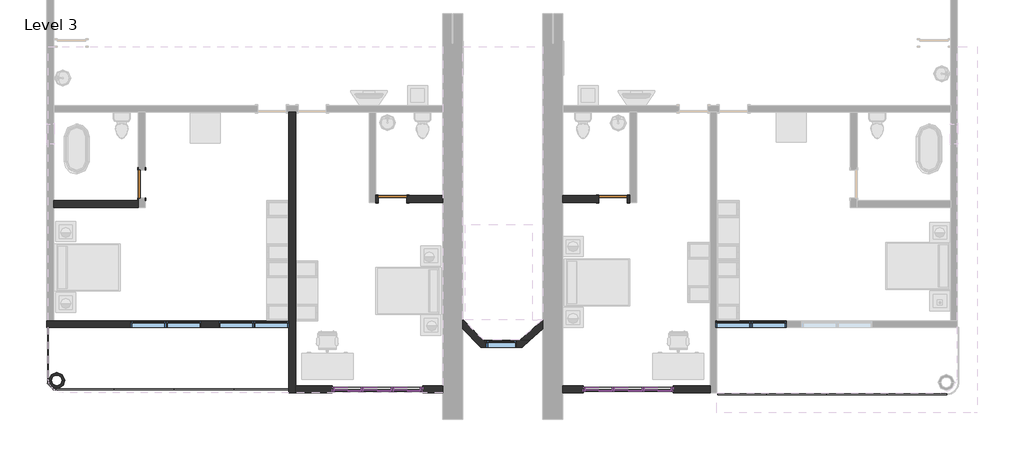
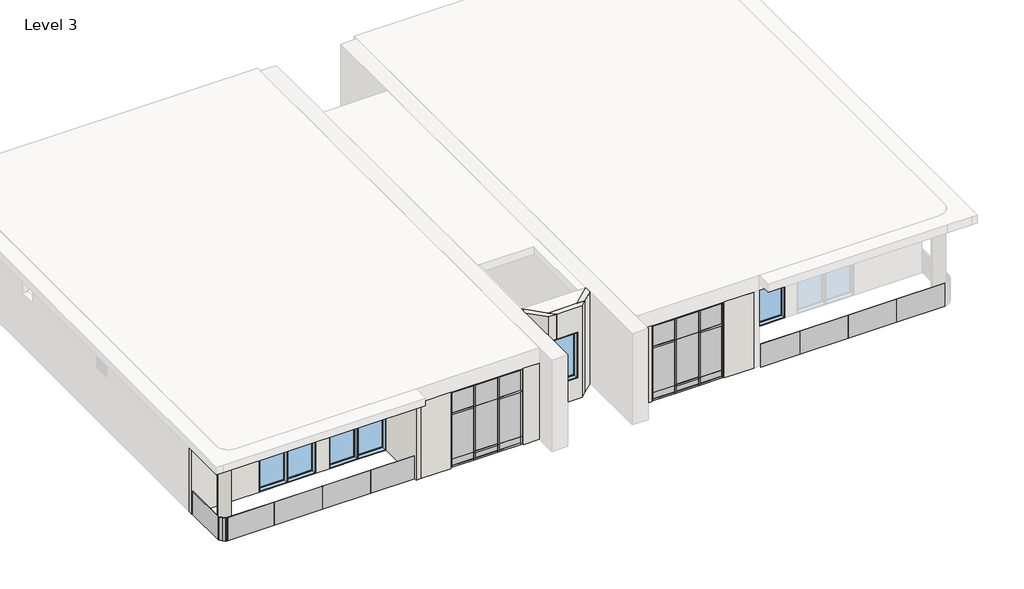
# One storey, part 1 of 3: 42 members, 31 plates, 14 walls, 7 windows, 3 doors.
"""IFC4 building model written with IfcOpenShell, lengths in millimetres."""

from ifc_helpers import new_model, si_unit, point, frame, frame_2d, origin, place, context, project, spatial, polyline, circle_curve, trimmed, segment, composite_curve, outline, extrude, faceted_brep, transform, mapped, element, save
from components import door_2703ae13, door_10fd3a06, member_c17f1be2, member_ad567e07, member_d2e7e466, member_7db1855a, member_75d1e245, member_d60e8053, member_3c3dc66a, member_2fae0574, member_410c6227, member_73c23c35, system_panel_glazed_38d54ecf, system_panel_glazed_fbb6c980, system_panel_glazed_4137532c, system_panel_glazed_6230de04, system_panel_glazed_a79f7f85, system_panel_glazed_9a5ea490, system_panel_glazed_95be5de7, system_panel_glazed_1e00a1c5, system_panel_glazed_ffe51582, system_panel_glazed_8f95e3f6, system_panel_glazed_836907cd, system_panel_glazed_688a65a2, system_panel_glazed_c1a1c740, system_panel_glazed_22bcd51f, window_9a779fa2, window_1a213a25

model = new_model("IFC4")

# Units and contexts
model_context = context("Model", 3, world=origin())
ifc_project = project(units=[si_unit("LENGTHUNIT", "METRE", prefix="MILLI")], contexts=[model_context])

# Site, building, storey
site = spatial("IfcSite", under=ifc_project)
building = spatial("IfcBuilding", under=site)
storey = spatial("IfcBuildingStorey", under=building, Name="Level 3", Elevation=7315.2)

# Doors
placement = place(None, origin())
door_shape = door_2703ae13(model_context)
element("IfcDoor", 1, ObjectType="Door-Single-Panel.0001 : 34\" x 80\"", at=placement, inside=storey, context=model_context, shape_type="MappedRepresentation", body=[
    mapped(door_shape, transform((-15759.6487704, -441.9241442, 7315.2), x_axis=(0.0, -1.0, 0.0), y_axis=(1.0, 0.0, 0.0), z_axis=(0.0, 0.0, 1.0))),
])
element("IfcDoor", 2, ObjectType="Door-Single-Panel.0001 : 34\" x 80\"", at=placement, inside=storey, context=model_context, shape_type="MappedRepresentation", body=[
    mapped(door_shape, transform((-8139.6487704, -899.1241442, 7315.2), x_axis=(-1.0, 0.0, 0.0), y_axis=(0.0, -1.0, 0.0), z_axis=(0.0, 0.0, 1.0))),
])
door_2_shape = door_10fd3a06(model_context)
element("IfcDoor", 3, ObjectType="Door-Single-Panel.0001 : 34\" x 80\"", at=placement, inside=storey, context=model_context, shape_type="MappedRepresentation", body=[
    mapped(door_2_shape, transform((-1434.0487704, -899.1241442, 7315.2), x_axis=(1.0, 0.0, 0.0), y_axis=(0.0, 1.0, 0.0), z_axis=(0.0, 0.0, 1.0))),
])

# Members
member_shape = member_c17f1be2(model_context)
element("IfcMember", 4, ObjectType="Rectangular Mullion : 2.5\" x 5\" rectangular", at=placement, inside=storey, context=model_context, shape_type="MappedRepresentation", body=[
    mapped(member_shape, transform((-9904.9487704, -6690.3241442, 10363.2), x_axis=(0.0, 0.0, 1.0), y_axis=(0.0, 1.0, 0.0), z_axis=(-1.0, 0.0, 0.0))),
])
element("IfcMember", 5, ObjectType="Rectangular Mullion : 2.5\" x 5\" rectangular", at=placement, inside=storey, context=model_context, shape_type="MappedRepresentation", body=[
    mapped(member_shape, transform((-8107.8987704, -6690.3241442, 10363.2), x_axis=(0.0, 0.0, 1.0), y_axis=(0.0, 1.0, 0.0), z_axis=(-1.0, 0.0, 0.0))),
])
element("IfcMember", 6, ObjectType="Rectangular Mullion : 2.5\" x 5\" rectangular", at=placement, inside=storey, context=model_context, shape_type="MappedRepresentation", body=[
    mapped(member_shape, transform((-2284.9487704, -6690.3241442, 10363.2), x_axis=(0.0, 0.0, 1.0), y_axis=(0.0, 1.0, 0.0), z_axis=(-1.0, 0.0, 0.0))),
])
element("IfcMember", 7, ObjectType="Rectangular Mullion : 2.5\" x 5\" rectangular", at=placement, inside=storey, context=model_context, shape_type="MappedRepresentation", body=[
    mapped(member_shape, transform((-487.8987704, -6690.3241442, 10363.2), x_axis=(0.0, 0.0, 1.0), y_axis=(0.0, 1.0, 0.0), z_axis=(-1.0, 0.0, 0.0))),
])
element("IfcMember", 8, ObjectType="Rectangular Mullion : 2.5\" x 5\" rectangular", at=placement, inside=storey, context=model_context, shape_type="MappedRepresentation", body=[
    mapped(member_shape, transform((-7288.7487704, -6690.3241442, 7315.2), x_axis=(0.0, 0.0, -1.0), y_axis=(0.0, 1.0, 0.0), z_axis=(1.0, 0.0, 0.0))),
])
element("IfcMember", 9, ObjectType="Rectangular Mullion : 2.5\" x 5\" rectangular", at=placement, inside=storey, context=model_context, shape_type="MappedRepresentation", body=[
    mapped(member_shape, transform((-9085.7987704, -6690.3241442, 7315.2), x_axis=(0.0, 0.0, -1.0), y_axis=(0.0, 1.0, 0.0), z_axis=(1.0, 0.0, 0.0))),
])
element("IfcMember", 10, ObjectType="Rectangular Mullion : 2.5\" x 5\" rectangular", at=placement, inside=storey, context=model_context, shape_type="MappedRepresentation", body=[
    mapped(member_shape, transform((331.2512296, -6690.3241442, 7315.2), x_axis=(0.0, 0.0, -1.0), y_axis=(0.0, 1.0, 0.0), z_axis=(1.0, 0.0, 0.0))),
])
element("IfcMember", 11, ObjectType="Rectangular Mullion : 2.5\" x 5\" rectangular", at=placement, inside=storey, context=model_context, shape_type="MappedRepresentation", body=[
    mapped(member_shape, transform((-1465.7987704, -6690.3241442, 7315.2), x_axis=(0.0, 0.0, -1.0), y_axis=(0.0, 1.0, 0.0), z_axis=(1.0, 0.0, 0.0))),
])
member_2_shape = member_ad567e07(model_context)
element("IfcMember", 12, ObjectType="Rectangular Mullion : 2.5\" x 5\" rectangular", at=placement, inside=storey, context=model_context, shape_type="MappedRepresentation", body=[
    mapped(member_2_shape, transform((-8107.8987704, -6690.3241442, 9448.8), x_axis=(0.0, 0.0, 1.0), y_axis=(0.0, 1.0, 0.0), z_axis=(-1.0, 0.0, 0.0))),
])
element("IfcMember", 13, ObjectType="Rectangular Mullion : 2.5\" x 5\" rectangular", at=placement, inside=storey, context=model_context, shape_type="MappedRepresentation", body=[
    mapped(member_2_shape, transform((-9904.9487704, -6690.3241442, 9448.8), x_axis=(0.0, 0.0, 1.0), y_axis=(0.0, 1.0, 0.0), z_axis=(-1.0, 0.0, 0.0))),
])
element("IfcMember", 14, ObjectType="Rectangular Mullion : 2.5\" x 5\" rectangular", at=placement, inside=storey, context=model_context, shape_type="MappedRepresentation", body=[
    mapped(member_2_shape, transform((-487.8987704, -6690.3241442, 9448.8), x_axis=(0.0, 0.0, 1.0), y_axis=(0.0, 1.0, 0.0), z_axis=(-1.0, 0.0, 0.0))),
])
element("IfcMember", 15, ObjectType="Rectangular Mullion : 2.5\" x 5\" rectangular", at=placement, inside=storey, context=model_context, shape_type="MappedRepresentation", body=[
    mapped(member_2_shape, transform((-2284.9487704, -6690.3241442, 9448.8), x_axis=(0.0, 0.0, 1.0), y_axis=(0.0, 1.0, 0.0), z_axis=(-1.0, 0.0, 0.0))),
])
member_3_shape = member_d2e7e466(model_context)
element("IfcMember", 16, ObjectType="Rectangular Mullion : 2.5\" x 5\" rectangular", at=placement, inside=storey, context=model_context, shape_type="MappedRepresentation", body=[
    mapped(member_3_shape, transform((-8171.3987704, -6690.3241442, 7315.2), x_axis=(0.0, 0.0, -1.0), y_axis=(0.0, 1.0, 0.0), z_axis=(1.0, 0.0, 0.0))),
])
element("IfcMember", 17, ObjectType="Rectangular Mullion : 2.5\" x 5\" rectangular", at=placement, inside=storey, context=model_context, shape_type="MappedRepresentation", body=[
    mapped(member_3_shape, transform((-551.3987704, -6690.3241442, 7315.2), x_axis=(0.0, 0.0, -1.0), y_axis=(0.0, 1.0, 0.0), z_axis=(1.0, 0.0, 0.0))),
])
member_4_shape = member_7db1855a(model_context)
element("IfcMember", 18, ObjectType="Rectangular Mullion : 2.5\" x 5\" rectangular", at=placement, inside=storey, context=model_context, shape_type="MappedRepresentation", body=[
    mapped(member_4_shape, transform((-9022.2987704, -6690.3241442, 7620.0), x_axis=(0.0, 0.0, 1.0), y_axis=(0.0, 1.0, 0.0), z_axis=(-1.0, 0.0, 0.0))),
])
element("IfcMember", 19, ObjectType="Rectangular Mullion : 2.5\" x 5\" rectangular", at=placement, inside=storey, context=model_context, shape_type="MappedRepresentation", body=[
    mapped(member_4_shape, transform((-1402.2987704, -6690.3241442, 7620.0), x_axis=(0.0, 0.0, 1.0), y_axis=(0.0, 1.0, 0.0), z_axis=(-1.0, 0.0, 0.0))),
])
element("IfcMember", 20, ObjectType="Rectangular Mullion : 2.5\" x 5\" rectangular", at=placement, inside=storey, context=model_context, shape_type="MappedRepresentation", body=[
    mapped(member_3_shape, transform((-9022.2987704, -6690.3241442, 10363.2), x_axis=(0.0, 0.0, 1.0), y_axis=(0.0, 1.0, 0.0), z_axis=(-1.0, 0.0, 0.0))),
])
element("IfcMember", 21, ObjectType="Rectangular Mullion : 2.5\" x 5\" rectangular", at=placement, inside=storey, context=model_context, shape_type="MappedRepresentation", body=[
    mapped(member_3_shape, transform((-1402.2987704, -6690.3241442, 10363.2), x_axis=(0.0, 0.0, 1.0), y_axis=(0.0, 1.0, 0.0), z_axis=(-1.0, 0.0, 0.0))),
])
member_5_shape = member_75d1e245(model_context)
element("IfcMember", 22, ObjectType="Rectangular Mullion : 2.5\" x 5\" rectangular", at=placement, inside=storey, context=model_context, shape_type="MappedRepresentation", body=[
    mapped(member_5_shape, transform((-8139.6487704, -6690.3241442, 7315.2), x_axis=(-1.0, 0.0, 0.0), y_axis=(0.0, 1.0, 0.0), z_axis=(0.0, 0.0, -1.0))),
])
element("IfcMember", 23, ObjectType="Rectangular Mullion : 2.5\" x 5\" rectangular", at=placement, inside=storey, context=model_context, shape_type="MappedRepresentation", body=[
    mapped(member_5_shape, transform((-9054.0487704, -6690.3241442, 7315.2), x_axis=(-1.0, 0.0, 0.0), y_axis=(0.0, 1.0, 0.0), z_axis=(0.0, 0.0, -1.0))),
])
element("IfcMember", 24, ObjectType="Rectangular Mullion : 2.5\" x 5\" rectangular", at=placement, inside=storey, context=model_context, shape_type="MappedRepresentation", body=[
    mapped(member_5_shape, transform((-519.6487704, -6690.3241442, 7315.2), x_axis=(-1.0, 0.0, 0.0), y_axis=(0.0, 1.0, 0.0), z_axis=(0.0, 0.0, -1.0))),
])
element("IfcMember", 25, ObjectType="Rectangular Mullion : 2.5\" x 5\" rectangular", at=placement, inside=storey, context=model_context, shape_type="MappedRepresentation", body=[
    mapped(member_5_shape, transform((-1434.0487704, -6690.3241442, 7315.2), x_axis=(-1.0, 0.0, 0.0), y_axis=(0.0, 1.0, 0.0), z_axis=(0.0, 0.0, -1.0))),
])
member_6_shape = member_d60e8053(model_context)
element("IfcMember", 26, ObjectType="Rectangular Mullion : 2.5\" x 5\" rectangular", at=placement, inside=storey, context=model_context, shape_type="MappedRepresentation", body=[
    mapped(member_6_shape, transform((-8139.6487704, -6690.3241442, 7620.0), x_axis=(-1.0, 0.0, 0.0), y_axis=(0.0, 1.0, 0.0), z_axis=(0.0, 0.0, -1.0))),
])
element("IfcMember", 27, ObjectType="Rectangular Mullion : 2.5\" x 5\" rectangular", at=placement, inside=storey, context=model_context, shape_type="MappedRepresentation", body=[
    mapped(member_6_shape, transform((-9054.0487704, -6690.3241442, 7620.0), x_axis=(-1.0, 0.0, 0.0), y_axis=(0.0, 1.0, 0.0), z_axis=(0.0, 0.0, -1.0))),
])
element("IfcMember", 28, ObjectType="Rectangular Mullion : 2.5\" x 5\" rectangular", at=placement, inside=storey, context=model_context, shape_type="MappedRepresentation", body=[
    mapped(member_6_shape, transform((-519.6487704, -6690.3241442, 7620.0), x_axis=(-1.0, 0.0, 0.0), y_axis=(0.0, 1.0, 0.0), z_axis=(0.0, 0.0, -1.0))),
])
element("IfcMember", 29, ObjectType="Rectangular Mullion : 2.5\" x 5\" rectangular", at=placement, inside=storey, context=model_context, shape_type="MappedRepresentation", body=[
    mapped(member_6_shape, transform((-1434.0487704, -6690.3241442, 7620.0), x_axis=(-1.0, 0.0, 0.0), y_axis=(0.0, 1.0, 0.0), z_axis=(0.0, 0.0, -1.0))),
])
member_7_shape = member_3c3dc66a(model_context)
element("IfcMember", 30, ObjectType="Rectangular Mullion : 2.5\" x 5\" rectangular", at=placement, inside=storey, context=model_context, shape_type="MappedRepresentation", body=[
    mapped(member_7_shape, transform((-9968.4487704, -6690.3241442, 7315.2), x_axis=(-1.0, 0.0, 0.0), y_axis=(0.0, 1.0, 0.0), z_axis=(0.0, 0.0, -1.0))),
])
element("IfcMember", 31, ObjectType="Rectangular Mullion : 2.5\" x 5\" rectangular", at=placement, inside=storey, context=model_context, shape_type="MappedRepresentation", body=[
    mapped(member_7_shape, transform((-2348.4487704, -6690.3241442, 7315.2), x_axis=(-1.0, 0.0, 0.0), y_axis=(0.0, 1.0, 0.0), z_axis=(0.0, 0.0, -1.0))),
])
member_8_shape = member_2fae0574(model_context)
element("IfcMember", 32, ObjectType="Rectangular Mullion : 2.5\" x 5\" rectangular", at=placement, inside=storey, context=model_context, shape_type="MappedRepresentation", body=[
    mapped(member_8_shape, transform((-9968.4487704, -6690.3241442, 7620.0), x_axis=(-1.0, 0.0, 0.0), y_axis=(0.0, 1.0, 0.0), z_axis=(0.0, 0.0, -1.0))),
])
element("IfcMember", 33, ObjectType="Rectangular Mullion : 2.5\" x 5\" rectangular", at=placement, inside=storey, context=model_context, shape_type="MappedRepresentation", body=[
    mapped(member_8_shape, transform((-2348.4487704, -6690.3241442, 7620.0), x_axis=(-1.0, 0.0, 0.0), y_axis=(0.0, 1.0, 0.0), z_axis=(0.0, 0.0, -1.0))),
])
element("IfcMember", 34, ObjectType="Rectangular Mullion : 2.5\" x 5\" rectangular", at=placement, inside=storey, context=model_context, shape_type="MappedRepresentation", body=[
    mapped(member_8_shape, transform((-7225.2487704, -6690.3241442, 9448.8), x_axis=(1.0, 0.0, 0.0), y_axis=(0.0, 1.0, 0.0), z_axis=(0.0, 0.0, 1.0))),
])
element("IfcMember", 35, ObjectType="Rectangular Mullion : 2.5\" x 5\" rectangular", at=placement, inside=storey, context=model_context, shape_type="MappedRepresentation", body=[
    mapped(member_8_shape, transform((394.7512296, -6690.3241442, 9448.8), x_axis=(1.0, 0.0, 0.0), y_axis=(0.0, 1.0, 0.0), z_axis=(0.0, 0.0, 1.0))),
])
element("IfcMember", 36, ObjectType="Rectangular Mullion : 2.5\" x 5\" rectangular", at=placement, inside=storey, context=model_context, shape_type="MappedRepresentation", body=[
    mapped(member_7_shape, transform((-7225.2487704, -6690.3241442, 7620.0), x_axis=(1.0, 0.0, 0.0), y_axis=(0.0, 1.0, 0.0), z_axis=(0.0, 0.0, 1.0))),
])
element("IfcMember", 37, ObjectType="Rectangular Mullion : 2.5\" x 5\" rectangular", at=placement, inside=storey, context=model_context, shape_type="MappedRepresentation", body=[
    mapped(member_7_shape, transform((394.7512296, -6690.3241442, 7620.0), x_axis=(1.0, 0.0, 0.0), y_axis=(0.0, 1.0, 0.0), z_axis=(0.0, 0.0, 1.0))),
])
member_9_shape = member_410c6227(model_context)
element("IfcMember", 38, ObjectType="Rectangular Mullion : 2.5\" x 5\" rectangular", at=placement, inside=storey, context=model_context, shape_type="MappedRepresentation", body=[
    mapped(member_9_shape, transform((-8139.6487704, -6690.3241442, 9448.8), x_axis=(-1.0, 0.0, 0.0), y_axis=(0.0, 1.0, 0.0), z_axis=(0.0, 0.0, -1.0))),
])
element("IfcMember", 39, ObjectType="Rectangular Mullion : 2.5\" x 5\" rectangular", at=placement, inside=storey, context=model_context, shape_type="MappedRepresentation", body=[
    mapped(member_9_shape, transform((-9054.0487704, -6690.3241442, 9448.8), x_axis=(-1.0, 0.0, 0.0), y_axis=(0.0, 1.0, 0.0), z_axis=(0.0, 0.0, -1.0))),
])
element("IfcMember", 40, ObjectType="Rectangular Mullion : 2.5\" x 5\" rectangular", at=placement, inside=storey, context=model_context, shape_type="MappedRepresentation", body=[
    mapped(member_9_shape, transform((-519.6487704, -6690.3241442, 9448.8), x_axis=(-1.0, 0.0, 0.0), y_axis=(0.0, 1.0, 0.0), z_axis=(0.0, 0.0, -1.0))),
])
element("IfcMember", 41, ObjectType="Rectangular Mullion : 2.5\" x 5\" rectangular", at=placement, inside=storey, context=model_context, shape_type="MappedRepresentation", body=[
    mapped(member_9_shape, transform((-1434.0487704, -6690.3241442, 9448.8), x_axis=(-1.0, 0.0, 0.0), y_axis=(0.0, 1.0, 0.0), z_axis=(0.0, 0.0, -1.0))),
])
member_10_shape = member_73c23c35(model_context)
element("IfcMember", 42, ObjectType="Rectangular Mullion : 2.5\" x 5\" rectangular", at=placement, inside=storey, context=model_context, shape_type="MappedRepresentation", body=[
    mapped(member_10_shape, transform((-7225.2487704, -6690.3241442, 10363.2), x_axis=(1.0, 0.0, 0.0), y_axis=(0.0, 1.0, 0.0), z_axis=(0.0, 0.0, 1.0))),
])
element("IfcMember", 43, ObjectType="Rectangular Mullion : 2.5\" x 5\" rectangular", at=placement, inside=storey, context=model_context, shape_type="MappedRepresentation", body=[
    mapped(member_10_shape, transform((394.7512296, -6690.3241442, 10363.2), x_axis=(1.0, 0.0, 0.0), y_axis=(0.0, 1.0, 0.0), z_axis=(0.0, 0.0, 1.0))),
])
element("IfcMember", 44, ObjectType="Rectangular Mullion : 2.5\" x 5\" rectangular", at=placement, inside=storey, context=model_context, shape_type="MappedRepresentation", body=[
    mapped(member_10_shape, transform((-9968.4487704, -6690.3241442, 9448.8), x_axis=(-1.0, 0.0, 0.0), y_axis=(0.0, 1.0, 0.0), z_axis=(0.0, 0.0, -1.0))),
])
element("IfcMember", 45, ObjectType="Rectangular Mullion : 2.5\" x 5\" rectangular", at=placement, inside=storey, context=model_context, shape_type="MappedRepresentation", body=[
    mapped(member_10_shape, transform((-2348.4487704, -6690.3241442, 9448.8), x_axis=(-1.0, 0.0, 0.0), y_axis=(0.0, 1.0, 0.0), z_axis=(0.0, 0.0, -1.0))),
])

# Plates
system_panel_glazed_shape = system_panel_glazed_38d54ecf(model_context)
element("IfcPlate", 46, ObjectType="System Panel : Glazed", at=placement, inside=storey, context=model_context, shape_type="MappedRepresentation", body=[
    mapped(system_panel_glazed_shape, transform((-8596.8487704, -6690.3241442, 7651.75), x_axis=(-1.0, 0.0, 0.0), y_axis=(0.0, -1.0, 0.0), z_axis=(0.0, 0.0, 1.0))),
])
element("IfcPlate", 47, ObjectType="System Panel : Glazed", at=placement, inside=storey, context=model_context, shape_type="MappedRepresentation", body=[
    mapped(system_panel_glazed_shape, transform((-976.8487704, -6690.3241442, 7651.75), x_axis=(-1.0, 0.0, 0.0), y_axis=(0.0, -1.0, 0.0), z_axis=(0.0, 0.0, 1.0))),
])
system_panel_glazed_2_shape = system_panel_glazed_fbb6c980(model_context)
element("IfcPlate", 48, ObjectType="System Panel : Glazed", at=placement, inside=storey, context=model_context, shape_type="MappedRepresentation", body=[
    mapped(system_panel_glazed_2_shape, transform((-8596.8487704, -6690.3241442, 7378.7), x_axis=(-1.0, 0.0, 0.0), y_axis=(0.0, -1.0, 0.0), z_axis=(0.0, 0.0, 1.0))),
])
element("IfcPlate", 49, ObjectType="System Panel : Glazed", at=placement, inside=storey, context=model_context, shape_type="MappedRepresentation", body=[
    mapped(system_panel_glazed_2_shape, transform((-976.8487704, -6690.3241442, 7378.7), x_axis=(-1.0, 0.0, 0.0), y_axis=(0.0, -1.0, 0.0), z_axis=(0.0, 0.0, 1.0))),
])
system_panel_glazed_3_shape = system_panel_glazed_4137532c(model_context)
element("IfcPlate", 50, ObjectType="System Panel : Glazed", at=placement, inside=storey, context=model_context, shape_type="MappedRepresentation", body=[
    mapped(system_panel_glazed_3_shape, transform((-7698.3237704, -6690.3241442, 7378.7), x_axis=(-1.0, 0.0, 0.0), y_axis=(0.0, -1.0, 0.0), z_axis=(0.0, 0.0, 1.0))),
])
element("IfcPlate", 51, ObjectType="System Panel : Glazed", at=placement, inside=storey, context=model_context, shape_type="MappedRepresentation", body=[
    mapped(system_panel_glazed_3_shape, transform((-9495.3737704, -6690.3241442, 7378.7), x_axis=(-1.0, 0.0, 0.0), y_axis=(0.0, -1.0, 0.0), z_axis=(0.0, 0.0, 1.0))),
])
element("IfcPlate", 52, ObjectType="System Panel : Glazed", at=placement, inside=storey, context=model_context, shape_type="MappedRepresentation", body=[
    mapped(system_panel_glazed_3_shape, transform((-78.3237704, -6690.3241442, 7378.7), x_axis=(-1.0, 0.0, 0.0), y_axis=(0.0, -1.0, 0.0), z_axis=(0.0, 0.0, 1.0))),
])
element("IfcPlate", 53, ObjectType="System Panel : Glazed", at=placement, inside=storey, context=model_context, shape_type="MappedRepresentation", body=[
    mapped(system_panel_glazed_3_shape, transform((-1875.3737704, -6690.3241442, 7378.7), x_axis=(-1.0, 0.0, 0.0), y_axis=(0.0, -1.0, 0.0), z_axis=(0.0, 0.0, 1.0))),
])
system_panel_glazed_4_shape = system_panel_glazed_6230de04(model_context)
element("IfcPlate", 54, ObjectType="System Panel : Glazed", at=placement, inside=storey, context=model_context, shape_type="MappedRepresentation", body=[
    mapped(system_panel_glazed_4_shape, transform((-7698.3237704, -6690.3241442, 7620.0), x_axis=(-1.0, 0.0, 0.0), y_axis=(0.0, -1.0, 0.0), z_axis=(0.0, 0.0, 1.0))),
])
element("IfcPlate", 55, ObjectType="System Panel : Glazed", at=placement, inside=storey, context=model_context, shape_type="MappedRepresentation", body=[
    mapped(system_panel_glazed_4_shape, transform((-9495.3737704, -6690.3241442, 7620.0), x_axis=(-1.0, 0.0, 0.0), y_axis=(0.0, -1.0, 0.0), z_axis=(0.0, 0.0, 1.0))),
])
element("IfcPlate", 56, ObjectType="System Panel : Glazed", at=placement, inside=storey, context=model_context, shape_type="MappedRepresentation", body=[
    mapped(system_panel_glazed_4_shape, transform((-78.3237704, -6690.3241442, 7620.0), x_axis=(-1.0, 0.0, 0.0), y_axis=(0.0, -1.0, 0.0), z_axis=(0.0, 0.0, 1.0))),
])
element("IfcPlate", 57, ObjectType="System Panel : Glazed", at=placement, inside=storey, context=model_context, shape_type="MappedRepresentation", body=[
    mapped(system_panel_glazed_4_shape, transform((-1875.3737704, -6690.3241442, 7620.0), x_axis=(-1.0, 0.0, 0.0), y_axis=(0.0, -1.0, 0.0), z_axis=(0.0, 0.0, 1.0))),
])
system_panel_glazed_5_shape = system_panel_glazed_a79f7f85(model_context)
element("IfcPlate", 58, ObjectType="System Panel : Glazed", at=placement, inside=storey, context=model_context, shape_type="MappedRepresentation", body=[
    mapped(system_panel_glazed_5_shape, transform((-7698.3237704, -6690.3241442, 9480.55), x_axis=(-1.0, 0.0, 0.0), y_axis=(0.0, -1.0, 0.0), z_axis=(0.0, 0.0, 1.0))),
])
element("IfcPlate", 59, ObjectType="System Panel : Glazed", at=placement, inside=storey, context=model_context, shape_type="MappedRepresentation", body=[
    mapped(system_panel_glazed_5_shape, transform((-9495.3737704, -6690.3241442, 9480.55), x_axis=(-1.0, 0.0, 0.0), y_axis=(0.0, -1.0, 0.0), z_axis=(0.0, 0.0, 1.0))),
])
element("IfcPlate", 60, ObjectType="System Panel : Glazed", at=placement, inside=storey, context=model_context, shape_type="MappedRepresentation", body=[
    mapped(system_panel_glazed_5_shape, transform((-78.3237704, -6690.3241442, 9480.55), x_axis=(-1.0, 0.0, 0.0), y_axis=(0.0, -1.0, 0.0), z_axis=(0.0, 0.0, 1.0))),
])
element("IfcPlate", 61, ObjectType="System Panel : Glazed", at=placement, inside=storey, context=model_context, shape_type="MappedRepresentation", body=[
    mapped(system_panel_glazed_5_shape, transform((-1875.3737704, -6690.3241442, 9480.55), x_axis=(-1.0, 0.0, 0.0), y_axis=(0.0, -1.0, 0.0), z_axis=(0.0, 0.0, 1.0))),
])
system_panel_glazed_6_shape = system_panel_glazed_9a5ea490(model_context)
element("IfcPlate", 62, ObjectType="System Panel : Glazed", at=placement, inside=storey, context=model_context, shape_type="MappedRepresentation", body=[
    mapped(system_panel_glazed_6_shape, transform((-8596.8487704, -6690.3241442, 9448.8), x_axis=(-1.0, 0.0, 0.0), y_axis=(0.0, -1.0, 0.0), z_axis=(0.0, 0.0, 1.0))),
])
element("IfcPlate", 63, ObjectType="System Panel : Glazed", at=placement, inside=storey, context=model_context, shape_type="MappedRepresentation", body=[
    mapped(system_panel_glazed_6_shape, transform((-976.8487704, -6690.3241442, 9448.8), x_axis=(-1.0, 0.0, 0.0), y_axis=(0.0, -1.0, 0.0), z_axis=(0.0, 0.0, 1.0))),
])
system_panel_glazed_7_shape = system_panel_glazed_95be5de7(model_context)
element("IfcPlate", 64, ObjectType="System Panel : Glazed", at=placement, inside=storey, context=model_context, shape_type="MappedRepresentation", body=[
    mapped(system_panel_glazed_7_shape, transform((-15700.8805745, -6723.6923401, 7315.2), x_axis=(1.0, 0.0, 0.0), y_axis=(0.0, 1.0, 0.0), z_axis=(0.0, 0.0, 1.0))),
])
element("IfcPlate", 65, ObjectType="System Panel : Glazed", at=placement, inside=storey, context=model_context, shape_type="MappedRepresentation", body=[
    mapped(system_panel_glazed_7_shape, transform((-13872.0805745, -6723.6923401, 7315.2), x_axis=(1.0, 0.0, 0.0), y_axis=(0.0, 1.0, 0.0), z_axis=(0.0, 0.0, 1.0))),
])
element("IfcPlate", 66, ObjectType="System Panel : Glazed", at=placement, inside=storey, context=model_context, shape_type="MappedRepresentation", body=[
    mapped(system_panel_glazed_7_shape, transform((7793.0620092, -6810.4133646, 7315.2), x_axis=(-1.0, 0.0, 0.0), y_axis=(0.0, -1.0, 0.0), z_axis=(0.0, 0.0, 1.0))),
])
element("IfcPlate", 67, ObjectType="System Panel : Glazed", at=placement, inside=storey, context=model_context, shape_type="MappedRepresentation", body=[
    mapped(system_panel_glazed_7_shape, transform((5964.2620092, -6810.4133646, 7315.2), x_axis=(-1.0, 0.0, 0.0), y_axis=(0.0, -1.0, 0.0), z_axis=(0.0, 0.0, 1.0))),
])
element("IfcPlate", 68, ObjectType="System Panel : Glazed", at=placement, inside=storey, context=model_context, shape_type="MappedRepresentation", body=[
    mapped(system_panel_glazed_7_shape, transform((4135.4620092, -6810.4133646, 7315.2), x_axis=(-1.0, 0.0, 0.0), y_axis=(0.0, -1.0, 0.0), z_axis=(0.0, 0.0, 1.0))),
])
system_panel_glazed_8_shape = system_panel_glazed_1e00a1c5(model_context)
element("IfcPlate", 69, ObjectType="System Panel : Glazed", at=placement, inside=storey, context=model_context, shape_type="MappedRepresentation", body=[
    mapped(system_panel_glazed_8_shape, transform((2484.4620092, -6810.4133646, 7315.2), x_axis=(-1.0, 0.0, 0.0), y_axis=(0.0, -1.0, 0.0), z_axis=(0.0, 0.0, 1.0))),
])
system_panel_glazed_9_shape = system_panel_glazed_ffe51582(model_context)
element("IfcPlate", 70, ObjectType="System Panel : Glazed", at=placement, inside=storey, context=model_context, shape_type="MappedRepresentation", body=[
    mapped(system_panel_glazed_9_shape, transform((-18445.6213429, -6722.1515718, 7315.2), x_axis=(0.7071067811865462, -0.7071067811865488, 0.0), y_axis=(0.7071067811865488, 0.7071067811865462, 0.0), z_axis=(0.0, 0.0, 1.0))),
])
system_panel_glazed_10_shape = system_panel_glazed_8f95e3f6(model_context)
element("IfcPlate", 71, ObjectType="System Panel : Glazed", at=placement, inside=storey, context=model_context, shape_type="MappedRepresentation", body=[
    mapped(system_panel_glazed_10_shape, transform((-18642.5487704, -5667.9741442, 7315.2), x_axis=(0.0, -1.0, 0.0), y_axis=(1.0, 0.0, 0.0), z_axis=(0.0, 0.0, 1.0))),
])
system_panel_glazed_11_shape = system_panel_glazed_836907cd(model_context)
element("IfcPlate", 72, ObjectType="System Panel : Glazed", at=placement, inside=storey, context=model_context, shape_type="MappedRepresentation", body=[
    mapped(system_panel_glazed_11_shape, transform((-18412.3305745, -6723.6923401, 7315.2), x_axis=(1.0, 0.0, 0.0), y_axis=(0.0, 1.0, 0.0), z_axis=(0.0, 0.0, 1.0))),
])
system_panel_glazed_12_shape = system_panel_glazed_688a65a2(model_context)
element("IfcPlate", 73, ObjectType="System Panel : Glazed", at=placement, inside=storey, context=model_context, shape_type="MappedRepresentation", body=[
    mapped(system_panel_glazed_12_shape, transform((-12123.4646725, -6723.6923401, 7315.2), x_axis=(1.0, 0.0, 0.0), y_axis=(0.0, 1.0, 0.0), z_axis=(0.0, 0.0, 1.0))),
])
system_panel_glazed_13_shape = system_panel_glazed_c1a1c740(model_context)
element("IfcPlate", 74, ObjectType="System Panel : Glazed", at=placement, inside=storey, context=model_context, shape_type="MappedRepresentation", body=[
    mapped(system_panel_glazed_13_shape, transform((-17497.9305745, -6723.6923401, 7315.2), x_axis=(1.0, 0.0, 0.0), y_axis=(0.0, 1.0, 0.0), z_axis=(0.0, 0.0, 1.0))),
])
system_panel_glazed_14_shape = system_panel_glazed_22bcd51f(model_context)
element("IfcPlate", 75, ObjectType="System Panel : Glazed", at=placement, inside=storey, context=model_context, shape_type="MappedRepresentation", body=[
    mapped(system_panel_glazed_14_shape, transform((-18593.7021056, -6574.070809, 7315.2), x_axis=(0.7071067811865462, -0.7071067811865488, 0.0), y_axis=(0.7071067811865488, 0.7071067811865462, 0.0), z_axis=(0.0, 0.0, 1.0))),
])
element("IfcPlate", 76, ObjectType="System Panel : Glazed", at=placement, inside=storey, context=model_context, shape_type="MappedRepresentation", body=[
    mapped(system_panel_glazed_14_shape, transform((-18496.0087761, -6671.7641386, 7315.2), x_axis=(0.7071067811865462, -0.7071067811865488, 0.0), y_axis=(0.7071067811865488, 0.7071067811865462, 0.0), z_axis=(0.0, 0.0, 1.0))),
])

# Walls
element("IfcWall", 77, ObjectType="Generic - 3\" green 2", at=placement, inside=storey, context=model_context, shape_type="SweptSolid", body=[
    extrude(outline(composite_curve([segment(polyline([(-18512.3737704, -6418.8616442), (-18588.5737704, -6418.8616442)]), True, "CONTINUOUS"), segment(trimmed(circle_curve(frame_2d((-18347.2737704, -6418.8616442)), 241.3), [point((-18588.5737704, -6418.8616442))], [point((-18105.9737704, -6418.8616442))], False, "CARTESIAN"), True, "CONTINUOUS"), segment(polyline([(-18105.9737704, -6418.8616442), (-18182.1737704, -6418.8616442)]), True, "CONTINUOUS"), segment(trimmed(circle_curve(frame_2d((-18347.2737704, -6418.8616442)), 165.1), [point((-18182.1737704, -6418.8616442))], [point((-18512.3737704, -6418.8616442))], True, "CARTESIAN"), True, "CONTINUOUS")], self_intersect=False)), frame((0.0, 0.0, 7315.2), z_axis=(0.0, 0.0, 1.0), x_axis=(1.0, 0.0, 0.0)), (0.0, 0.0, 1.0), 3048.0),
])
element("IfcWall", 78, ObjectType="Generic - 3\" green 2", at=placement, inside=storey, context=model_context, shape_type="SweptSolid", body=[
    extrude(outline(composite_curve([segment(polyline([(-18182.1737704, -6418.8616442), (-18105.9737704, -6418.8616442)]), True, "CONTINUOUS"), segment(trimmed(circle_curve(frame_2d((-18347.2737704, -6418.8616442)), 241.3), [point((-18105.9737704, -6418.8616442))], [point((-18588.5737704, -6418.8616442))], False, "CARTESIAN"), True, "CONTINUOUS"), segment(polyline([(-18588.5737704, -6418.8616442), (-18512.3737704, -6418.8616442)]), True, "CONTINUOUS"), segment(trimmed(circle_curve(frame_2d((-18347.2737704, -6418.8616442)), 165.1), [point((-18512.3737704, -6418.8616442))], [point((-18182.1737704, -6418.8616442))], True, "CARTESIAN"), True, "CONTINUOUS")], self_intersect=False)), frame((0.0, 0.0, 7315.2), z_axis=(0.0, 0.0, 1.0), x_axis=(1.0, 0.0, 0.0)), (0.0, 0.0, 1.0), 3048.0),
])
element("IfcWall", 79, ObjectType="Generic - 8\" cream", at=placement, inside=storey, context=model_context, shape_type="Brep", body=[
    faceted_brep([(-11289.2487704, 1742.4758558, 7315.2), (-11289.2487704, -6791.9241442, 7315.2), (-11289.2487704, -6791.9241442, 10363.2), (-11289.2487704, -4810.7241442, 10363.2), (-11289.2487704, -4607.5241442, 10363.2), (-11289.2487704, 1742.4758558, 10363.2), (-11086.0487704, 1742.4758558, 7315.2), (-11086.0487704, 1742.4758558, 10363.2), (-11086.0487704, -6588.7241442, 10363.2), (-11086.0487704, -6791.9241442, 10363.2), (-11086.0487704, -6791.9241442, 7315.2), (-11086.0487704, -6588.7241442, 7315.2)], [[[0, 1, 2, 3, 4, 5]], [[6, 7, 8, 9, 10, 11]], [[1, 0, 6, 11, 10]], [[5, 4, 3, 2, 9, 8, 7]], [[0, 5, 7, 6]], [[2, 1, 10, 9]]]),
])
element("IfcWall", 80, ObjectType="Generic - 8\" cream", at=placement, inside=storey, context=model_context, shape_type="SweptSolid", body=[
    extrude(outline(polyline([(-18439.3487704, -949.9241442), (-15861.2487704, -949.9241442), (-15861.2487704, -1153.1241442), (-18439.3487704, -1153.1241442), (-18439.3487704, -949.9241442)])), frame((0.0, 0.0, 7315.2), z_axis=(0.0, 0.0, 1.0), x_axis=(1.0, 0.0, 0.0)), (0.0, 0.0, 1.0), 3048.0),
])
element("IfcWall", 81, ObjectType="Generic - 8\" cream", at=placement, inside=storey, context=model_context, shape_type="SweptSolid", body=[
    extrude(outline(polyline([(10363.2, -6615.6487704), (10363.2, -8647.6487704), (7315.2, -8647.6487704), (7315.2, -8571.4487704), (9347.2, -8571.4487704), (9347.2, -7707.8487704), (7315.2, -7707.8487704), (7315.2, -6615.6487704), (10363.2, -6615.6487704)])), frame((0.0, -1000.7241442, 0.0), z_axis=(0.0, 1.0, 0.0), x_axis=(0.0, 0.0, 1.0)), (0.0, 0.0, 1.0), 203.2),
])
element("IfcWall", 82, ObjectType="Generic - 8\" cream", at=placement, inside=storey, context=model_context, shape_type="Brep", body=[
    faceted_brep([(-18642.5487704, -4607.5241442, 10363.2), (-18439.3487704, -4607.5241442, 10363.2), (-11289.2487704, -4607.5241442, 10363.2), (-11289.2487704, -4607.5241442, 10058.4), (-13422.8487704, -4607.5241442, 10058.4), (-13422.8487704, -4607.5241442, 7315.2), (-13956.2487704, -4607.5241442, 7315.2), (-13956.2487704, -4607.5241442, 10058.4), (-16089.8487704, -4607.5241442, 10058.4), (-16089.8487704, -4607.5241442, 7315.2), (-18439.3487704, -4607.5241442, 7315.2), (-18642.5487704, -4607.5241442, 7315.2), (-11289.2487704, -4810.7241442, 10363.2), (-18642.5487704, -4810.7241442, 10363.2), (-18642.5487704, -4810.7241442, 7315.2), (-16089.8487704, -4810.7241442, 7315.2), (-16089.8487704, -4810.7241442, 10058.4), (-13956.2487704, -4810.7241442, 10058.4), (-13956.2487704, -4810.7241442, 7315.2), (-13422.8487704, -4810.7241442, 7315.2), (-13422.8487704, -4810.7241442, 10058.4), (-11289.2487704, -4810.7241442, 10058.4)], [[[0, 1, 2, 3, 4, 5, 6, 7, 8, 9, 10, 11]], [[12, 13, 14, 15, 16, 17, 18, 19, 20, 21]], [[14, 11, 10, 9, 15]], [[5, 19, 18, 6]], [[2, 1, 0, 13, 12]], [[2, 12, 21, 3]], [[0, 11, 14, 13]], [[3, 21, 20, 4]], [[4, 20, 19, 5]], [[17, 7, 6, 18]], [[7, 17, 16, 8]], [[8, 16, 15, 9]]]),
])
element("IfcWall", 83, ObjectType="Generic - 8\" cream", at=placement, inside=storey, context=model_context, shape_type="SweptSolid", body=[
    extrude(outline(polyline([(10363.2, -926.0487704), (10363.2, -2958.0487704), (7315.2, -2958.0487704), (7315.2, -1865.8487704), (9347.2, -1865.8487704), (9347.2, -1002.2487704), (7315.2, -1002.2487704), (7315.2, -926.0487704), (10363.2, -926.0487704)])), frame((0.0, -1000.7241442, 0.0), z_axis=(0.0, 1.0, 0.0), x_axis=(0.0, 0.0, 1.0)), (0.0, 0.0, 1.0), 203.2),
])
element("IfcWall", 84, ObjectType="Generic - 8\" cream", at=placement, inside=storey, context=model_context, shape_type="SweptSolid", body=[
    extrude(outline(polyline([(394.7512296, -6588.7241442), (1512.3512296, -6588.7241442), (1512.3512296, -6791.9241442), (394.7512296, -6791.9241442), (394.7512296, -6588.7241442)])), frame((0.0, 0.0, 7315.2), z_axis=(0.0, 0.0, 1.0), x_axis=(1.0, 0.0, 0.0)), (0.0, 0.0, 1.0), 3048.0),
])
element("IfcWall", 85, ObjectType="Generic - 8\" cream", at=placement, inside=storey, context=model_context, shape_type="SweptSolid", body=[
    extrude(outline(polyline([(-2348.4487704, -6791.9241442), (-2958.0487704, -6791.9241442), (-2958.0487704, -6588.7241442), (-2348.4487704, -6588.7241442), (-2348.4487704, -6791.9241442)])), frame((0.0, 0.0, 7315.2), z_axis=(0.0, 0.0, 1.0), x_axis=(1.0, 0.0, 0.0)), (0.0, 0.0, 1.0), 3048.0),
])
element("IfcWall", 86, ObjectType="Generic - 8\" cream", at=placement, inside=storey, context=model_context, shape_type="SweptSolid", body=[
    extrude(outline(polyline([(-9968.4487704, -6791.9241442), (-11086.0487704, -6791.9241442), (-11086.0487704, -6588.7241442), (-9968.4487704, -6588.7241442), (-9968.4487704, -6791.9241442)])), frame((0.0, 0.0, 7315.2), z_axis=(0.0, 0.0, 1.0), x_axis=(1.0, 0.0, 0.0)), (0.0, 0.0, 1.0), 3048.0),
])
element("IfcWall", 87, ObjectType="Generic - 8\" cream", at=placement, inside=storey, context=model_context, shape_type="SweptSolid", body=[
    extrude(outline(polyline([(-7225.2487704, -6588.7241442), (-6615.6487704, -6588.7241442), (-6615.6487704, -6791.9241442), (-7225.2487704, -6791.9241442), (-7225.2487704, -6588.7241442)])), frame((0.0, 0.0, 7315.2), z_axis=(0.0, 0.0, 1.0), x_axis=(1.0, 0.0, 0.0)), (0.0, 0.0, 1.0), 3048.0),
])
element("IfcWall", 88, ObjectType="Generic - 8\" green", at=placement, inside=storey, context=model_context, shape_type="Brep", body=[
    faceted_brep([(-6006.0487704, -4852.8082422, 7315.2), (-5452.3544276, -5406.502585, 7315.2), (-5452.3544276, -5406.502585, 10972.8), (-6006.0487704, -4852.8082422, 10972.8), (-5164.9862318, -5406.502585, 7315.2), (-5368.1862318, -5203.302585, 7315.2), (-6006.0487704, -4565.4400463, 7315.2), (-6006.0487704, -4565.4400463, 10972.8), (-5368.1862318, -5203.302585, 10972.8), (-5164.9862318, -5406.502585, 10972.8), (-5164.9862318, -5406.502585, 9982.2), (-5283.1401401, -5288.3486766, 9982.2), (-5283.1401401, -5288.3486766, 8153.4), (-5164.9862318, -5406.502585, 8153.4), (-5283.1401401, -5406.502585, 8153.4), (-5283.1401401, -5406.502585, 9982.2)], [[[0, 1, 2, 3]], [[4, 5, 6, 7, 8, 9, 10, 11, 12, 13]], [[1, 0, 6, 5, 4]], [[3, 2, 9, 8, 7]], [[0, 3, 7, 6]], [[2, 1, 4, 13, 14, 15, 10, 9]], [[12, 14, 13]], [[14, 12, 11, 15]], [[15, 11, 10]]]),
])
element("IfcWall", 89, ObjectType="Generic - 8\" green", at=placement, inside=storey, context=model_context, shape_type="Brep", body=[
    faceted_brep([(-5164.9862318, -5406.502585, 7315.2), (-4196.9843712, -5406.502585, 7315.2), (-4196.9843712, -5406.502585, 10972.8), (-5164.9862318, -5406.502585, 10972.8), (-5164.9862318, -5406.502585, 9982.2), (-4368.7401401, -5406.502585, 9982.2), (-4368.7401401, -5406.502585, 8153.4), (-5164.9862318, -5406.502585, 8153.4), (-3969.1320774, -5203.302585, 7315.2), (-4274.4301413, -5203.302585, 7315.2), (-5368.1862318, -5203.302585, 7315.2), (-5368.1862318, -5203.302585, 10972.8), (-4274.4301413, -5203.302585, 10972.8), (-3969.1320774, -5203.302585, 10972.8), (-4368.7401401, -5203.302585, 8153.4), (-4368.7401401, -5203.302585, 9982.2), (-5283.1401401, -5203.302585, 9982.2), (-5283.1401401, -5203.302585, 8153.4), (-5283.1401401, -5288.3486766, 8153.4), (-5283.1401401, -5288.3486766, 9982.2)], [[[0, 1, 2, 3, 4, 5, 6, 7]], [[8, 9, 10, 11, 12, 13], [14, 15, 16, 17]], [[1, 0, 10, 9, 8]], [[3, 2, 13, 12, 11]], [[3, 11, 10, 0, 7, 18, 19, 4]], [[2, 1, 8, 13]], [[5, 15, 14, 6]], [[6, 14, 17, 18, 7]], [[18, 17, 16, 19]], [[15, 5, 4, 19, 16]]]),
])
element("IfcWall", 90, ObjectType="Generic - 8\" green", at=placement, inside=storey, context=model_context, shape_type="SweptSolid", body=[
    extrude(outline(polyline([(-3567.6487704, -4845.2574382), (-3969.1320774, -5203.302585), (-4274.4301413, -5203.302585), (-3567.6487704, -4572.9908503), (-3567.6487704, -4845.2574382)])), frame((0.0, 0.0, 7315.2), z_axis=(0.0, 0.0, 1.0), x_axis=(1.0, 0.0, 0.0)), (0.0, 0.0, 1.0), 3657.6),
])

# Windows
window_shape = window_9a779fa2(model_context)
element("IfcWindow", 91, ObjectType="Fixed : 36\" x 72\"", at=placement, inside=storey, context=model_context, shape_type="MappedRepresentation", body=[
    mapped(window_shape, transform((-4787.8401401, -5304.902585, 7848.6), x_axis=(1.0, 0.0, 0.0), y_axis=(0.0, 1.0, 0.0), z_axis=(0.0, 0.0, 1.0))),
])
window_2_shape = window_1a213a25(model_context)
element("IfcWindow", 92, ObjectType="Fixed : 36\" x 72\" 2", at=placement, inside=storey, context=model_context, shape_type="MappedRepresentation", body=[
    mapped(window_2_shape, transform((-11784.5487704, -4709.1241442, 7010.4), x_axis=(1.0, 0.0, 0.0), y_axis=(0.0, 1.0, 0.0), z_axis=(0.0, 0.0, 1.0))),
])
element("IfcWindow", 93, ObjectType="Fixed : 36\" x 72\" 2", at=placement, inside=storey, context=model_context, shape_type="MappedRepresentation", body=[
    mapped(window_2_shape, transform((-12851.3487704, -4709.1241442, 7010.4), x_axis=(1.0, 0.0, 0.0), y_axis=(0.0, 1.0, 0.0), z_axis=(0.0, 0.0, 1.0))),
])
element("IfcWindow", 94, ObjectType="Fixed : 36\" x 72\" 2", at=placement, inside=storey, context=model_context, shape_type="MappedRepresentation", body=[
    mapped(window_2_shape, transform((-14451.5487704, -4709.1241442, 7010.4), x_axis=(1.0, 0.0, 0.0), y_axis=(0.0, 1.0, 0.0), z_axis=(0.0, 0.0, 1.0))),
])
element("IfcWindow", 95, ObjectType="Fixed : 36\" x 72\" 2", at=placement, inside=storey, context=model_context, shape_type="MappedRepresentation", body=[
    mapped(window_2_shape, transform((-15518.3487704, -4709.1241442, 7010.4), x_axis=(1.0, 0.0, 0.0), y_axis=(0.0, 1.0, 0.0), z_axis=(0.0, 0.0, 1.0))),
])
element("IfcWindow", 96, ObjectType="Fixed : 36\" x 72\" 2", at=placement, inside=storey, context=model_context, shape_type="MappedRepresentation", body=[
    mapped(window_2_shape, transform((2261.6512296, -4709.1241442, 7010.4), x_axis=(1.0, 0.0, 0.0), y_axis=(0.0, 1.0, 0.0), z_axis=(0.0, 0.0, 1.0))),
])
element("IfcWindow", 97, ObjectType="Fixed : 36\" x 72\" 2", at=placement, inside=storey, context=model_context, shape_type="MappedRepresentation", body=[
    mapped(window_2_shape, transform((3337.9762296, -4709.1241442, 7010.4), x_axis=(1.0, 0.0, 0.0), y_axis=(0.0, 1.0, 0.0), z_axis=(0.0, 0.0, 1.0))),
])

save(model, "model.ifc")

# Revit data of these elements
# Type "Door-Single-Panel.0001 : 34\" x 80\""
#   Type Mark = "9"
#   Construction Type Id = "DOOR"
#   Assembly Code = "C1020300"
#   Analytic Construction = "Wooden"
#   Thickness = 0' - 2"
#   Thermal Resistance (R) = 0.455703 (m²·K)/W
#   Swing Angle [instance default] = 90.00°
#   Heat Transfer Coefficient (U) = 2.19465 W/(m²·K)
#   Height = 6' - 8"
#   Trim Projection Ext = 0' - 1"
#   Trim Projection Int = 0' - 1"
#   Trim Width = 0' - 3"
#   Width = 2' - 10"
#   Panel Material = Wood - Birch - Solid Stained Light Low Gloss
#   Trim Material = Paint - Sienna
#   Visual Light Transmittance = 0
#   Solar Heat Gain Coefficient = 0
#   Function = (empty or 0)
#   Wall Closure = (empty or 0)
# Type "Rectangular Mullion : 2.5\" x 5\" rectangular"
#   built-in parameter 1007304 = 0.416667 (stored number, unit not read)
#   built-in parameter 1007301 = 0.104167 (stored number, unit not read)
#   built-in parameter 1007300 = 0.104167 (stored number, unit not read)
# Type "System Panel : Glazed"
#   Construction Type Id = "GSP4R"
#   Analytic Construction = "1/8 in Pilkington single glazing"
#   Visual Light Transmittance = 0.9
#   Solar Heat Gain Coefficient = 0.86
#   Heat Transfer Coefficient (U) = 6.7069 W/(m²·K)
# Type "Generic - 3\" green 2"
#   Assembly Code = "B2010"
#   Width = 0' - 3"
#   Layers, outside or top first: 0' - 3" "Damp-proofing" (function 1)
# Type "Generic - 8\" cream"
#   Assembly Code = "B2010"
#   Width = 0' - 8"
#   Layers, outside or top first: 0' - 8" "Parking Stripe" (function 1)
# Type "Generic - 8\" green"
#   Assembly Code = "B2010"
#   Width = 0' - 8"
#   Layers, outside or top first: 0' - 8" "Damp-proofing" (function 1)
# Type "Fixed : 36\" x 72\""
#   Type Mark = "9"
#   Construction Type Id = "GSP4R"
#   Assembly Code = "B2020100"
#   Analytic Construction = "1/8 in Pilkington single glazing"
#   Visual Light Transmittance = 0.9
#   Solar Heat Gain Coefficient = 0.78
#   Heat Transfer Coefficient (U) = 3.6886 W/(m²·K)
#   Height = 6' - 0"
#   Default Sill Height = 1' - 0"
#   Width = 3' - 0"
#   Window Inset = 0' - 0 3/4"
#   Glass Pane Material = Glass
#   Sash Material = Iron, Ductile
#   Wall Closure = (empty or 0)
# Type "Fixed : 36\" x 72\" 2"
#   Type Mark = "29"
#   Construction Type Id = "GSP4R"
#   Assembly Code = "B2020100"
#   Analytic Construction = "1/8 in Pilkington single glazing"
#   Visual Light Transmittance = 0.9
#   Solar Heat Gain Coefficient = 0.78
#   Heat Transfer Coefficient (U) = 3.6886 W/(m²·K)
#   Height = 9' - 0"
#   Default Sill Height = 1' - 0"
#   Width = 3' - 6"
#   Window Inset = 0' - 0 3/4"
#   Glass Pane Material = Glass
#   Sash Material = Iron, Ductile
#   Wall Closure = (empty or 0)
# Elements 1, 2, 3 (IfcDoor, "Door-Single-Panel.0001 : 34\" x 80\"")
#   Swing Angle = 90.00°
#   Phase Created = New Construction
#   Materials on its faces: "Paint - Sienna", "Wood - Birch - Solid Stained Light Low Gloss"
# Elements 4, 5, 6, 7, 8, 9, 10, 11, 12, 13, 14, 15, 16, 17, 18, 19, 20, 21, 22, 23, 24, 25, 26, 27, 28, 29, 30, 31, 32, 33, 34, 35, 36, 37, 38, 39, 40, 41, 42, 43, 44, 45 (IfcMember, "Rectangular Mullion : 2.5\" x 5\" rectangular")
#   Phase Created = New Construction
#   Materials on its faces: "Iron, Ductile"
# Elements 46, 47, 48, 49, 50, 51, 52, 53, 54, 55, 56, 57, 58, 59, 60, 61, 62, 63, 64, 65, 66, 67, 68, 69, 70, 71, 72, 73, 74, 75, 76 (IfcPlate, "System Panel : Glazed")
#   Phase Created = New Construction
#   Materials on its faces: "Glass"
# Elements 77, 78 (IfcWall, "Generic - 3\" green 2")
#   Top Offset = 0' - 0"
#   Base Offset = 0' - 0"
#   Unconnected Height = 10' - 0"
#   wall height = 10' - 0"
#   Phase Created = New Construction
#   Materials on its faces: "Damp-proofing"
# Elements 79, 80, 81, 82, 83, 84, 85, 86, 87 (IfcWall, "Generic - 8\" cream")
#   Top Offset = 0' - 0"
#   Base Offset = 0' - 0"
#   Unconnected Height = 10' - 0"
#   wall height = 10' - 0"
#   Phase Created = New Construction
#   Base Constraint = Level 3
#   Materials on its faces: "Parking Stripe"
# Elements 88, 89, 90 (IfcWall, "Generic - 8\" green")
#   Top Offset = 0' - 0"
#   Base Offset = 0' - 0"
#   Unconnected Height = 12' - 0"
#   wall height = 12' - 0"
#   Phase Created = New Construction
#   Base Constraint = Level 3
#   Materials on its faces: "Damp-proofing"
# Element 91 (IfcWindow, "Fixed : 36\" x 72\"")
#   Mark = "93"
#   Phase Created = New Construction
#   Materials on its faces: "Iron, Ductile", "Glass"
# Element 92 (IfcWindow, "Fixed : 36\" x 72\" 2")
#   Mark = "94"
#   Phase Created = New Construction
#   Materials on its faces: "Iron, Ductile", "Glass"
# Element 93 (IfcWindow, "Fixed : 36\" x 72\" 2")
#   Mark = "95"
#   Phase Created = New Construction
#   Materials on its faces: "Iron, Ductile", "Glass"
# Element 94 (IfcWindow, "Fixed : 36\" x 72\" 2")
#   Mark = "96"
#   Phase Created = New Construction
#   Materials on its faces: "Iron, Ductile", "Glass"
# Element 95 (IfcWindow, "Fixed : 36\" x 72\" 2")
#   Mark = "97"
#   Phase Created = New Construction
#   Materials on its faces: "Iron, Ductile", "Glass"
# Element 96 (IfcWindow, "Fixed : 36\" x 72\" 2")
#   Mark = "98"
#   Phase Created = New Construction
#   Materials on its faces: "Iron, Ductile", "Glass"
# Element 97 (IfcWindow, "Fixed : 36\" x 72\" 2")
#   Mark = "99"
#   Phase Created = New Construction
#   Materials on its faces: "Iron, Ductile", "Glass"
# Materials
#   "Wood - Birch - Solid Stained Light Low Gloss": class "Wood", colour RGB 210 159 95, transparency 0, Cost = 0
#   "Paint - Sienna": colour RGB 118 70 51, transparency 0, Cost = 0
#   "Damp-proofing": class "Generic", colour RGB 127 127 127, transparency 0, Description = "Damp-proofing", Cost = 0
#   "Parking Stripe": class "Paint", colour RGB 250 250 91, transparency 0, Cost = 0
#   "Glass": class "Glass", colour RGB 0 128 192, transparency 0.75, Description = "Soda Lime Glass", Cost = 0
#   "Iron, Ductile": class "Metal", colour RGB 0 0 0, transparency 0, Description = "Ductile cast iron", Cost = 0
